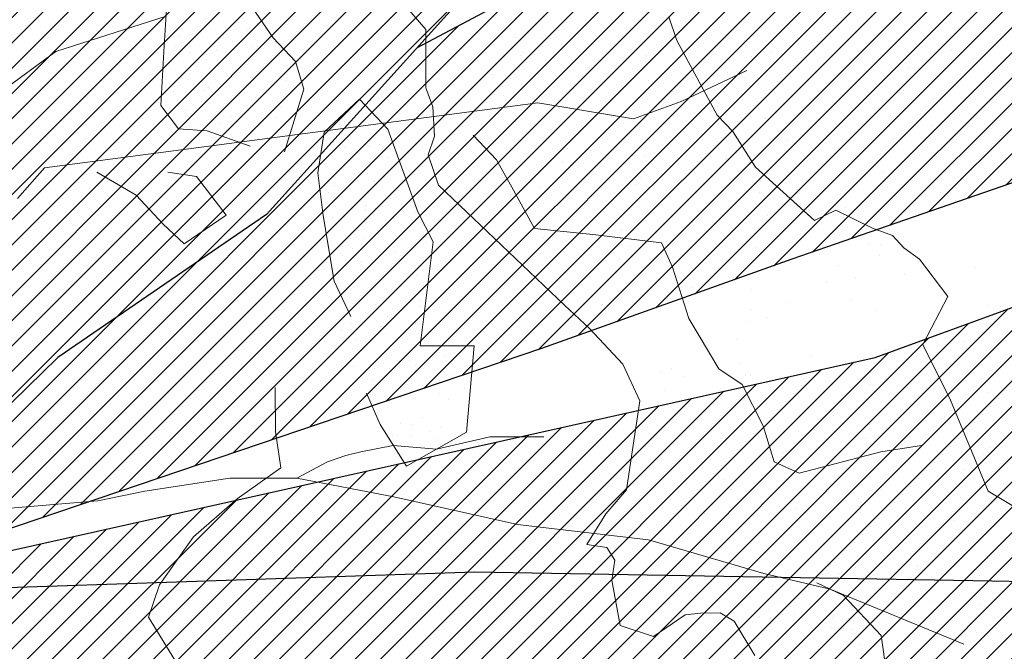
# Model space of a CAD drawing. Units: inches. Extents: x 1986 to 21484, y -1816 to 2016.
# Tile 70 of 85: x 3670.627 to 3679.11, y 1883.347 to 1888.787. Entities that reach past the tile are written whole.
import ezdxf

# ---------------------------------------------------------------- set-up
doc = ezdxf.new("R2010")
doc.units = ezdxf.units.IN
doc.layers.add('L-PLNT', color=84, linetype='Continuous', lineweight=13)
doc.layers.add('vfolhas', color=114, linetype='Continuous', lineweight=5)
doc.layers.add('vfolha2', color=110, linetype='Continuous')
doc.layers.add('vfolhas2', color=102, linetype='Continuous')
pattern_1 = [(45, (-2446.5133113, 50.986076), (-0.004419417382, 0.004419417382), [])]

# ---------------------------------------------------------------- blocks, each defined once
blk = doc.blocks.new('arbusto_PB_verde_grande')
at = {"layer": 'vfolha2'}
h = blk.add_hatch(dxfattribs=at)
h.set_pattern_fill('ANSI31', color=256, scale=0.05, style=0)
h.set_pattern_definition(pattern_1)
h.paths.add_polyline_path([(0.02944, 0.35651), (0.00028, 0.09048), (0.02625, -0.03934), (0.047, 0.06233), (0.06189, 0.09731), (0.09372, 0.26573), (0.09955, 0.43473), (0.08789, 0.61313), (0.0645, 0.72266), (0.04988, 0.6851), (0.0236, 0.51294)])
h.paths.add_polyline_path([(0.30106, 0.43789), (0.14225, 0.24871), (0.26685, 0.30022)])
h.paths.add_polyline_path([(0.37995, 0.22817), (0.23697, 0.15193), (0.18428, 0.09364), (0.11122, 0.04358), (0.02625, -0.03934), (0.28061, 0.04667), (0.36829, 0.07798), (0.46756, 0.11239), (0.61068, 0.19376), (0.71585, 0.27823), (0.55813, 0.25948)])
h.paths.add_polyline_path([(0.56101, -0.29441), (0.72752, -0.32573), (0.59024, -0.2412), (0.42962, -0.15982), (0.02625, -0.03934), (0.14922, -0.14107), (0.18838, -0.16604), (0.41501, -0.24435)])
h.paths.add_polyline_path([(-0.27429, -0.44776), (-0.30352, -0.72628), (-0.23923, -0.64175), (-0.15457, -0.45716), (0.02625, -0.03934), (-0.16328, -0.25376)])
h.paths.add_polyline_path([(-0.51963, -0.24744), (-0.67736, -0.32573), (-0.59558, -0.35072), (-0.40574, -0.32882), (-0.21007, -0.20995), (0.02625, -0.03934), (-0.14874, -0.06595), (-0.31518, -0.09101), (-0.41452, -0.15048)])
h.paths.add_polyline_path([(-0.52546, 0.25007), (-0.70947, 0.24698), (-0.51963, 0.1093), (-0.32979, 0.02167), (-0.07567, -0.0128), (-0.04234, -0.02148), (-0.35024, 0.1312)])
at = {"layer": 'vfolhas'}
h = blk.add_hatch(dxfattribs=at)
h.set_pattern_fill('ANSI31', color=256, scale=0.05, style=0)
h.set_pattern_definition(pattern_1)
h.paths.add_polyline_path([(-0.07279, 0.50669), (-0.18085, 0.65063), (-0.2334, 0.67253), (-0.20712, 0.53176), (-0.10785, 0.25007), (0.02625, -0.03934), (0.00028, 0.09048), (0.00816, 0.16241), (-0.04939, 0.29079)])
h.paths.add_polyline_path([(0.09902, 0.41929), (0.09372, 0.26573), (0.07906, 0.18814), (0.15506, 0.36901), (0.26606, 0.5505), (0.28356, 0.63504), (0.2485, 0.68819), (0.25145, 0.63504), (0.20178, 0.54426)])
h.paths.add_polyline_path([(0.12295, 0.24073), (0.047, 0.06233), (0.02625, -0.03934), (0.11122, 0.04358), (0.18428, 0.09364), (0.27478, 0.19376), (0.3215, 0.25323), (0.44129, 0.38467), (0.47634, 0.57866), (0.41789, 0.45347), (0.28939, 0.30954)])
h.paths.add_polyline_path([(0.58145, -0.03779), (0.70707, 0.01536), (0.78591, 0.04667), (0.74796, 0.06549), (0.62818, 0.08423), (0.52595, 0.09048), (0.39745, 0.04358), (0.02625, -0.03934), (0.25728, -0.03154), (0.43834, -0.0347)])
h.paths.add_polyline_path([(0.52022, -0.03647), (0.43834, -0.0347), (0.25728, -0.03154), (0.02625, -0.03934), (0.17964, -0.08515), (0.53768, -0.13167), (0.69541, -0.15357), (0.78591, -0.07852), (0.70413, -0.10042)])
h.paths.add_polyline_path([(0.27189, -0.21929), (0.14922, -0.14107), (0.02625, -0.03934), (0.15794, -0.31007), (0.29522, -0.42585), (0.41789, -0.49157), (0.56396, -0.56669), (0.5114, -0.48532), (0.39456, -0.34139)])
h.paths.add_polyline_path([(-0.05818, -0.47591), (-0.02312, -0.61984), (0.047, -0.80134), (0.08494, -0.59794), (0.07911, -0.4071), (0.03527, -0.25376), (0.02625, -0.03934), (-0.03773, -0.26001)])
h.paths.add_polyline_path([(-0.24218, 0.14054), (-0.11073, 0.06858), (0.02625, -0.03934), (-0.04235, 0.10871), (-0.21007, 0.23757), (-0.36485, 0.33145), (-0.47874, 0.40341), (-0.54303, 0.46288), (-0.49041, 0.33145), (-0.39408, 0.22192)])
at = {"layer": 'vfolha2'}
for p, q in [((0.23697, 0.15193), (0.37995, 0.22817)), ((0.36829, 0.07798), (0.28061, 0.04667)), ((0.28061, 0.04667), (0.02625, -0.03934))]:
    blk.add_line(p, q, dxfattribs=at)
at = {"layer": 'vfolhas2'}
for p, q in [((0.27478, 0.19376), (0.18428, 0.09364)), ((0.46756, 0.11239), (0.36829, 0.07798)), ((0.18428, 0.09364), (0.11122, 0.04358)), ((0.39745, 0.04358), (0.52595, 0.09048)), ((0.02625, -0.03934), (0.39745, 0.04358)), ((0.11122, 0.04358), (0.02625, -0.03934)), ((0.25728, -0.03154), (0.02625, -0.03934)), ((0.43834, -0.0347), (0.25728, -0.03154)), ((0.58145, -0.03779), (0.43834, -0.0347))]:
    blk.add_line(p, q, dxfattribs=at)
blk = doc.blocks.new('PLANT-SHRUB')
for p, q in [((2157.0668, 1897.0355), (2157.0668, 1897.0355)), ((2157.0784, 1897.0518), (2157.0784, 1897.0518)), ((2157.224, 1897.0515), (2157.739, 1895.9176)), ((2156.8868, 1896.8951), (2156.8868, 1896.8951)), ((2157.4297, 1896.8237), (2157.4297, 1896.8237)), ((2157.6934, 1896.5097), (2157.9487, 1896.8741)), ((2156.5712, 1896.6515), (2156.5712, 1896.6515)), ((2156.6455, 1896.6493), (2156.6455, 1896.6493)), ((2156.7191, 1896.7168), (2156.7191, 1896.7168)), ((2157.159, 1896.6045), (2157.159, 1896.6045)), ((2157.6174, 1896.6382), (2157.6174, 1896.6382)), ((2156.1686, 1896.2344), (2156.0761, 1896.5528)), ((2157.6934, 1896.036), (2157.6934, 1896.5097)), ((2157.875, 1896.4405), (2157.875, 1896.4405)), ((2157.9206, 1896.3661), (2157.9206, 1896.3661)), ((2157.9206, 1896.3661), (2157.9206, 1896.3661)), ((2155.8693, 1895.4412), (2156.1686, 1896.2344)), ((2156.0308, 1896.2768), (2156.0308, 1896.2768)), ((2156.2476, 1896.2848), (2156.2476, 1896.2848)), ((2157.0532, 1896.2817), (2157.0532, 1896.2817)), ((2157.8469, 1896.2986), (2157.8469, 1896.2986)), ((2157.8469, 1896.2986), (2157.8469, 1896.2986)), ((2157.8874, 1896.246), (2157.8874, 1896.246)), ((2157.9914, 1896.2323), (2157.9914, 1896.2323)), ((2158.0927, 1896.2986), (2158.0927, 1896.2986)), ((2158.1327, 1896.2428), (2158.1327, 1896.2428)), ((2158.1327, 1896.2428), (2158.1327, 1896.2428)), ((2158.1327, 1896.2428), (2158.1327, 1896.2428)), ((2156.5523, 1896.218), (2156.5523, 1896.218)), ((2157.7969, 1896.2157), (2157.7969, 1896.2157)), ((2157.7969, 1896.2157), (2157.7969, 1896.2157)), ((2157.9584, 1896.162), (2157.9584, 1896.162)), ((2158.1538, 1896.2109), (2158.1538, 1896.2109)), ((2156.3837, 1896.1106), (2156.3837, 1896.1106)), ((2157.6284, 1896.1083), (2157.6284, 1896.1083)), ((2157.8624, 1896.0555), (2157.8624, 1896.0555)), ((2157.8742, 1896.1083), (2157.8742, 1896.1083)), ((2157.8938, 1896.1163), (2157.8938, 1896.1163)), ((2155.9854, 1895.979), (2155.9854, 1895.979)), ((2157.7846, 1895.7991), (2157.6934, 1896.036)), ((2155.8263, 1895.8987), (2155.8263, 1895.8987)), ((2155.8999, 1895.9662), (2155.8999, 1895.9662)), ((2156.1934, 1895.9516), (2156.1934, 1895.9516)), ((2156.5183, 1895.9088), (2156.5183, 1895.9088)), ((2157.4491, 1895.934), (2157.4491, 1895.934)), ((2157.739, 1895.9176), (2158.063, 1895.429)), ((2158.4945, 1895.9409), (2158.4945, 1895.9409)), ((2158.5295, 1895.5526), (2158.6031, 1895.8917)), ((2156.5461, 1895.8815), (2156.5461, 1895.8815)), ((2157.0612, 1895.8374), (2157.0612, 1895.8374)), ((2157.2692, 1895.81), (2157.2692, 1895.81)), ((2157.5922, 1895.8681), (2157.5922, 1895.8681)), ((2158.1004, 1895.8549), (2158.1004, 1895.8549)), ((2158.1201, 1895.8578), (2158.1201, 1895.8578)), ((2157.5941, 1895.7672), (2157.5941, 1895.7672)), ((2157.9696, 1895.7178), (2157.9696, 1895.7178)), ((2158.2839, 1895.7478), (2158.2839, 1895.7478)), ((2158.3207, 1895.7816), (2158.3207, 1895.7816)), ((2158.137, 1895.6957), (2158.137, 1895.6957)), ((2158.137, 1895.6957), (2158.137, 1895.6957)), ((2158.241, 1895.682), (2158.241, 1895.682)), ((2158.345, 1895.6683), (2158.345, 1895.6683)), ((2158.345, 1895.6683), (2158.345, 1895.6683)), ((2158.345, 1895.6683), (2158.345, 1895.6683)), ((2158.3611, 1895.6729), (2158.3611, 1895.6729)), ((2158.4193, 1895.6605), (2158.4193, 1895.6605)), ((2158.5075, 1895.647), (2158.5075, 1895.647)), ((2155.5916, 1895.606), (2155.5916, 1895.606)), ((2156.32, 1895.5542), (2156.6117, 1895.3538)), ((2156.8362, 1895.6037), (2156.8362, 1895.6037)), ((2157.0277, 1895.5479), (2157.0277, 1895.5479)), ((2157.1014, 1895.6154), (2157.1014, 1895.6154)), ((2158.0809, 1895.6014), (2158.0809, 1895.6014)), ((2158.0809, 1895.6014), (2158.0809, 1895.6014)), ((2158.085, 1895.5656), (2158.085, 1895.5656)), ((2158.3351, 1895.6068), (2158.3351, 1895.6068)), ((2158.5691, 1895.4169), (2158.5295, 1895.5526)), ((2155.4285, 1895.5342), (2155.4285, 1895.5342)), ((2156.0056, 1895.5067), (2156.0056, 1895.5067)), ((2157.028, 1895.5116), (2157.028, 1895.5116)), ((2158.1075, 1895.4727), (2158.1075, 1895.4727)), ((2158.1075, 1895.4727), (2158.1075, 1895.4727)), ((2158.1075, 1895.4727), (2158.1075, 1895.4727)), ((2155.7151, 1894.9276), (2155.8693, 1895.4412)), ((2158.063, 1895.429), (2158.5889, 1894.5368)), ((2158.6936, 1895.3039), (2158.5691, 1895.4169)), ((2156.6117, 1895.3538), (2157.2499, 1895.0076)), ((2158.8011, 1895.2247), (2158.6936, 1895.3039)), ((2155.0808, 1895.2156), (2155.0808, 1895.2156)), ((2156.2295, 1895.2172), (2156.2295, 1895.2172)), ((2157.4741, 1895.2149), (2157.4741, 1895.2149)), ((2158.3029, 1895.2646), (2158.3029, 1895.2646)), ((2158.3029, 1895.2646), (2158.3029, 1895.2646)), ((2158.3485, 1895.2878), (2158.3485, 1895.2878)), ((2159.1292, 1895.1739), (2158.8011, 1895.2247)), ((2155.0071, 1895.1481), (2155.0071, 1895.1481)), ((2155.4414, 1895.1502), (2155.4414, 1895.1502)), ((2156.6299, 1895.1834), (2156.6299, 1895.1834)), ((2158.2292, 1895.1971), (2158.2292, 1895.1971)), ((2158.2292, 1895.1971), (2158.2292, 1895.1971)), ((2158.258, 1895.1601), (2158.258, 1895.1601)), ((2158.3232, 1895.1538), (2158.3232, 1895.1538)), ((2158.475, 1895.1971), (2158.475, 1895.1971)), ((2159.1292, 1895.1739), (2159.1292, 1895.1739)), ((2159.2706, 1894.9082), (2159.1292, 1895.1739)), ((2155.074, 1895.0642), (2155.074, 1895.0642)), ((2156.0609, 1895.1098), (2156.0609, 1895.1098)), ((2156.5209, 1895.1114), (2156.5209, 1895.1114)), ((2157.3056, 1895.1075), (2157.3056, 1895.1075)), ((2157.5671, 1895.098), (2157.5671, 1895.098)), ((2155.6169, 1894.9927), (2155.6169, 1894.9927)), ((2155.8249, 1894.9653), (2155.8249, 1894.9653)), ((2157.2499, 1895.0076), (2157.3411, 1894.7889)), ((2155.2731, 1894.7735), (2155.7151, 1894.9276)), ((2155.7151, 1894.9276), (2155.7151, 1894.9276)), ((2156.1498, 1894.9225), (2156.1498, 1894.9225)), ((2159.0575, 1894.575), (2159.2706, 1894.9082)), ((2156.2086, 1894.7973), (2156.2086, 1894.7973)), ((2156.2822, 1894.8648), (2156.2822, 1894.8648)), ((2156.6927, 1894.8511), (2156.6927, 1894.8511)), ((2156.9007, 1894.8237), (2156.9007, 1894.8237)), ((2157.3411, 1894.7889), (2157.1952, 1894.4974)), ((2157.8314, 1894.8326), (2157.8314, 1894.8326)), ((2154.9343, 1894.75), (2154.9343, 1894.75)), ((2155.232, 1894.373), (2155.2731, 1894.7735)), ((2155.9804, 1894.7366), (2155.9804, 1894.7366)), ((2157.0028, 1894.7415), (2157.0028, 1894.7415)), ((2157.2256, 1894.7809), (2157.2256, 1894.7809)), ((2157.7685, 1894.7094), (2157.7685, 1894.7094)), ((2158.0823, 1894.7026), (2158.0823, 1894.7026)), ((2157.9765, 1894.6821), (2157.9765, 1894.6821)), ((2158.3015, 1894.6393), (2158.3015, 1894.6393)), ((2155.2688, 1894.6051), (2155.2688, 1894.6051)), ((2156.5134, 1894.6029), (2156.5134, 1894.6029)), ((2157.7581, 1894.6006), (2157.7581, 1894.6006)), ((2158.5889, 1894.5368), (2159.3227, 1893.6692)), ((2158.9216, 1894.4663), (2159.0575, 1894.575)), ((2157.1952, 1894.4974), (2157.0858, 1894.1148)), ((2157.41, 1894.4465), (2157.41, 1894.4465)), ((2157.4837, 1894.514), (2157.4837, 1894.514)), ((2158.8944, 1894.3395), (2158.9216, 1894.4663)), ((2154.3938, 1894.3752), (2154.3938, 1894.3752)), ((2155.2628, 1894.2086), (2155.232, 1894.373)), ((2155.4162, 1894.3802), (2155.4162, 1894.3802)), ((2155.8108, 1894.4328), (2155.8108, 1894.4328)), ((2156.4957, 1894.3413), (2156.4957, 1894.3413)), ((2157.5419, 1894.3279), (2157.5419, 1894.3279)), ((2159.0031, 1894.2037), (2158.8944, 1894.3395)), ((2154.6621, 1894.2186), (2154.6621, 1894.2186)), ((2155.2628, 1894.0648), (2155.2628, 1894.2086)), ((2155.9067, 1894.2163), (2155.9067, 1894.2163)), ((2157.1513, 1894.2141), (2157.1513, 1894.2141)), ((2158.7041, 1894.1222), (2159.0031, 1894.2037)), ((2154.1725, 1894.148), (2154.1725, 1894.148)), ((2154.3806, 1894.1207), (2154.3806, 1894.1207)), ((2154.4935, 1894.1112), (2154.4935, 1894.1112)), ((2155.463, 1894.1141), (2155.463, 1894.1141)), ((2155.7382, 1894.109), (2155.7382, 1894.109)), ((2156.9828, 1894.1067), (2156.9828, 1894.1067)), ((2157.0858, 1894.1148), (2157.1405, 1893.878)), ((2158.4322, 1894.0951), (2158.7041, 1894.1222)), ((2154.7055, 1894.0779), (2154.7055, 1894.0779)), ((2155.3451, 1893.9005), (2155.2628, 1894.0648)), ((2155.3894, 1894.0466), (2155.3894, 1894.0466)), ((2157.0122, 1894.082), (2157.0122, 1894.082)), ((2157.8249, 1893.6131), (2158.4322, 1894.0951)), ((2154.9091, 1893.9799), (2154.9091, 1893.9799)), ((2155.2484, 1894.0064), (2155.2484, 1894.0064)), ((2155.4564, 1893.979), (2155.4564, 1893.979)), ((2155.7813, 1893.9362), (2155.7813, 1893.9362)), ((2155.9553, 1893.9665), (2155.9553, 1893.9665)), ((2156.9777, 1893.9714), (2156.9777, 1893.9714)), ((2155.4684, 1893.5718), (2155.3451, 1893.9005)), ((2156.3242, 1893.8648), (2156.3242, 1893.8648)), ((2157.1405, 1893.878), (2157.0311, 1893.386)), ((2158.0571, 1893.9325), (2158.0571, 1893.9325)), ((2156.5322, 1893.8374), (2156.5322, 1893.8374)), ((2156.8571, 1893.7946), (2156.8571, 1893.7946)), ((2154.9916, 1893.6821), (2154.9916, 1893.6821)), ((2156.5908, 1893.6959), (2156.5908, 1893.6959)), ((2156.6645, 1893.7634), (2156.6645, 1893.7634)), ((2157.4, 1893.7231), (2157.4, 1893.7231)), ((2157.608, 1893.6958), (2157.608, 1893.6958)), ((2153.7014, 1893.6066), (2153.7014, 1893.6066)), ((2154.3687, 1893.6052), (2154.3687, 1893.6052)), ((2154.946, 1893.6043), (2154.946, 1893.6043)), ((2155.3911, 1893.6101), (2155.3911, 1893.6101)), ((2156.1906, 1893.6021), (2156.1906, 1893.6021)), ((2157.4353, 1893.5998), (2157.4353, 1893.5998)), ((2157.7148, 1893.2832), (2157.8249, 1893.6131)), ((2157.8249, 1893.6131), (2157.8249, 1893.6131)), ((2157.933, 1893.653), (2157.933, 1893.653)), ((2159.3227, 1893.6692), (2159.9342, 1892.7649)), ((2155.4684, 1893.5718), (2155.4684, 1893.5718)), ((2155.6637, 1893.5102), (2155.4684, 1893.5718)), ((2155.7187, 1892.8278), (2155.6637, 1893.5102)), ((2156.4705, 1893.5712), (2156.4705, 1893.5712)), ((2157.5167, 1893.5578), (2157.5167, 1893.5578)), ((2154.6439, 1893.3635), (2154.6439, 1893.3635)), ((2157.0311, 1893.386), (2156.8305, 1892.967)), ((2154.5702, 1893.296), (2154.5702, 1893.296)), ((2156.193, 1893.3313), (2156.193, 1893.3313)), ((2157.7148, 1893.2832), (2157.7148, 1893.2832)), ((2157.7148, 1892.8616), (2157.7148, 1893.2832)), ((2158.6395, 1893.2743), (2158.9777, 1892.9557)), ((2153.8045, 1893.2487), (2153.8045, 1893.2487)), ((2154.3393, 1893.2178), (2154.3393, 1893.2178)), ((2154.8839, 1893.2098), (2154.8839, 1893.2098)), ((2155.5839, 1893.2155), (2155.5839, 1893.2155)), ((2155.9301, 1893.1964), (2155.9301, 1893.1964)), ((2156.8285, 1893.2133), (2156.8285, 1893.2133)), ((2156.9525, 1893.2013), (2156.9525, 1893.2013)), ((2154.1707, 1893.1104), (2154.1707, 1893.1104)), ((2155.4154, 1893.1082), (2155.4154, 1893.1082)), ((2156.66, 1893.1059), (2156.66, 1893.1059)), ((2155.8453, 1893.0127), (2155.8453, 1893.0127)), ((2154.1724, 1892.9315), (2154.1724, 1892.9315)), ((2155.7717, 1892.9452), (2155.7717, 1892.9452)), ((2156.8305, 1892.967), (2156.7576, 1892.7483)), ((2157.3945, 1892.9806), (2157.3945, 1892.9806)), ((2158.9777, 1892.9557), (2159.3871, 1892.7184)), ((2154.3435, 1892.8351), (2154.3435, 1892.8351)), ((2155.3659, 1892.84), (2155.3659, 1892.84)), ((2157.7331, 1892.5683), (2157.7148, 1892.8616)), ((2155.6536, 1892.4702), (2155.7187, 1892.8278)), ((2156.4454, 1892.8011), (2156.4454, 1892.8011)), ((2156.7576, 1892.7483), (2157.1223, 1892.3111)), ((2157.4915, 1892.7877), (2157.4915, 1892.7877)), ((2158.5418, 1892.2911), (2159.0987, 1892.788)), ((2159.0987, 1892.788), (2159.6754, 1892.6488)), ((2159.9342, 1892.7649), (2160.4349, 1892.0769)), ((2157.0468, 1892.6619), (2157.0468, 1892.6619)), ((2159.3871, 1892.7184), (2159.6357, 1892.4402)), ((2154.6232, 1892.6035), (2154.6232, 1892.6035)), ((2155.3739, 1892.5807), (2155.3739, 1892.5807)), ((2155.8679, 1892.6013), (2155.8679, 1892.6013)), ((2156.9731, 1892.5944), (2156.9731, 1892.5944)), ((2157.1125, 1892.599), (2157.1125, 1892.599)), ((2159.2337, 1892.601), (2159.2337, 1892.601)), ((2159.3179, 1892.6547), (2159.3179, 1892.6547)), ((2159.6754, 1892.6488), (2159.5959, 1892.2315)), ((2159.6754, 1892.6488), (2159.6754, 1892.6488)), ((2157.8167, 1891.0729), (2157.7331, 1892.5683)), ((2158.8533, 1892.497), (2158.8533, 1892.497)), ((2159.3232, 1892.5664), (2159.3232, 1892.5664)), ((2162.2835, 1892.5519), (2162.1841, 1892.075)), ((2154.8587, 1892.4397), (2154.8587, 1892.4397)), ((2155.6536, 1892.2751), (2155.6536, 1892.4702)), ((2155.9049, 1892.4263), (2155.9049, 1892.4263)), ((2156.9273, 1892.4312), (2156.9273, 1892.4312)), ((2159.0157, 1892.4756), (2159.0157, 1892.4756)), ((2159.2872, 1892.4399), (2159.2872, 1892.4399)), ((2159.3912, 1892.4262), (2159.3912, 1892.4262)), ((2159.4307, 1892.4436), (2159.4307, 1892.4436)), ((2159.4675, 1892.4773), (2159.4675, 1892.4773)), ((2159.6357, 1892.4402), (2159.8763, 1892.2895)), ((2158.8376, 1892.3486), (2158.8376, 1892.3486)), ((2159.0411, 1892.3881), (2159.0411, 1892.3881)), ((2159.4599, 1892.3475), (2159.4599, 1892.3475)), ((2159.5537, 1892.4048), (2159.5537, 1892.4048)), ((2159.5808, 1892.3687), (2159.5808, 1892.3687)), ((2155.0262, 1892.2621), (2155.0262, 1892.2621)), ((2155.4666, 1891.568), (2155.6536, 1892.2751)), ((2157.1223, 1892.3111), (2157.4687, 1891.9102)), ((2158.8799, 1891.9731), (2158.5418, 1892.2911)), ((2159.2318, 1892.2613), (2159.2318, 1892.2613)), ((2159.8763, 1892.2895), (2159.9923, 1892.2219)), ((2154.9525, 1892.1946), (2154.9525, 1892.1946)), ((2155.7995, 1891.9784), (2155.2052, 1892.1705)), ((2155.2611, 1892.2147), (2155.2611, 1892.2147)), ((2156.5058, 1892.2125), (2156.5058, 1892.2125)), ((2156.5753, 1892.2299), (2156.5753, 1892.2299)), ((2157.7504, 1892.2102), (2157.7504, 1892.2102)), ((2158.7875, 1892.188), (2158.7875, 1892.188)), ((2159.1565, 1892.1542), (2159.1565, 1892.1542)), ((2159.3106, 1892.1813), (2159.3106, 1892.1813)), ((2159.5959, 1892.2315), (2159.4964, 1891.9533)), ((2159.9923, 1892.2219), (2160.1469, 1892.1543)), ((2160.1469, 1892.1543), (2160.4349, 1892.0769)), ((2155.0926, 1892.1073), (2155.0926, 1892.1073)), ((2155.3407, 1892.0699), (2155.3407, 1892.0699)), ((2156.3372, 1892.1051), (2156.3372, 1892.1051)), ((2157.5818, 1892.1028), (2157.5818, 1892.1028)), ((2159.0211, 1892.0683), (2159.0211, 1892.0683)), ((2159.0579, 1892.102), (2159.0579, 1892.102)), ((2159.0723, 1892.1006), (2159.0723, 1892.1006)), ((2160.4349, 1892.0769), (2160.8561, 1891.6818)), ((2162.1841, 1892.075), (2161.9255, 1891.9359)), ((2156.4202, 1892.031), (2156.4202, 1892.031)), ((2157.4663, 1892.0176), (2157.4663, 1892.0176)), ((2159.0285, 1892.0031), (2159.0285, 1892.0031)), ((2155.0443, 1891.9637), (2155.0443, 1891.9637)), ((2156.2016, 1891.8037), (2155.7995, 1891.9784)), ((2156.2276, 1891.9113), (2156.2276, 1891.9113)), ((2157.4687, 1891.9102), (2157.3776, 1891.5458)), ((2158.1838, 1891.3968), (2158.8799, 1891.9731)), ((2159.1029, 1891.9467), (2159.1029, 1891.9467)), ((2159.2069, 1891.933), (2159.2069, 1891.933)), ((2159.3694, 1891.9117), (2159.3694, 1891.9117)), ((2160.4737, 1891.916), (2160.2947, 1891.6576)), ((2160.9311, 1891.8564), (2160.4737, 1891.916)), ((2161.9255, 1891.9359), (2161.4283, 1891.8365)), ((2155.5872, 1891.8922), (2155.5872, 1891.8922)), ((2155.7952, 1891.8648), (2155.7952, 1891.8648)), ((2156.1202, 1891.822), (2156.1202, 1891.822)), ((2156.1539, 1891.8438), (2156.1539, 1891.8438)), ((2158.8222, 1891.886), (2158.8222, 1891.886)), ((2159.2985, 1891.8471), (2159.2985, 1891.8471)), ((2161.4283, 1891.8365), (2160.9311, 1891.8564)), ((2156.7085, 1891.14), (2156.2016, 1891.8037)), ((2156.663, 1891.7506), (2156.663, 1891.7506)), ((2158.7749, 1891.8029), (2158.7749, 1891.8029)), ((2159.298, 1891.7963), (2159.298, 1891.7963)), ((2155.8797, 1891.6562), (2155.8797, 1891.6562)), ((2156.8711, 1891.7232), (2156.8711, 1891.7232)), ((2156.9021, 1891.6611), (2156.9021, 1891.6611)), ((2157.196, 1891.6804), (2157.196, 1891.6804)), ((2158.6115, 1891.6929), (2158.6115, 1891.6929)), ((2158.6484, 1891.7267), (2158.6484, 1891.7267)), ((2158.9952, 1891.6538), (2158.9952, 1891.6538)), ((2159.4229, 1891.7106), (2159.4229, 1891.7106)), ((2160.2947, 1891.6576), (2160.0361, 1891.3794)), ((2160.8561, 1891.6818), (2161.4664, 1891.2609)), ((2155.3771, 1891.3729), (2155.4666, 1891.568)), ((2155.5451, 1891.6004), (2155.5451, 1891.6004)), ((2156.7897, 1891.5982), (2156.7897, 1891.5982)), ((2157.4291, 1891.5605), (2157.4291, 1891.5605)), ((2158.5047, 1891.6156), (2158.5047, 1891.6156)), ((2158.9109, 1891.6001), (2158.9109, 1891.6001)), ((2159.0159, 1891.618), (2159.0159, 1891.618)), ((2155.7561, 1891.4793), (2155.7561, 1891.4793)), ((2157.3776, 1891.5458), (2157.3046, 1891.2543)), ((2157.3554, 1891.493), (2157.3554, 1891.493)), ((2158.3808, 1891.5244), (2158.3808, 1891.5244)), ((2158.4126, 1891.5107), (2158.4126, 1891.5107)), ((2158.4848, 1891.5107), (2158.4848, 1891.5107)), ((2158.6472, 1891.4893), (2158.6472, 1891.4893)), ((2159.2123, 1891.5176), (2159.2123, 1891.5176)), ((2159.2491, 1891.5513), (2159.2491, 1891.5513)), ((2158.1042, 1891.1186), (2158.1838, 1891.3968)), ((2158.7623, 1891.4179), (2158.7623, 1891.4179)), ((2158.9187, 1891.4536), (2158.9187, 1891.4536)), ((2159.0227, 1891.4399), (2159.0227, 1891.4399)), ((2159.1852, 1891.4185), (2159.1852, 1891.4185)), ((2159.2854, 1891.4112), (2159.2854, 1891.4112)), ((2158.2019, 1891.3176), (2158.2019, 1891.3176)), ((2158.2388, 1891.3514), (2158.2388, 1891.3514)), ((2158.5148, 1891.3478), (2158.5148, 1891.3478)), ((2159.0134, 1891.3353), (2159.0134, 1891.3353)), ((2159.1411, 1891.3794), (2159.039, 1891.059)), ((2159.4566, 1891.3828), (2159.4566, 1891.3828)), ((2156.395, 1891.2609), (2156.395, 1891.2609)), ((2157.3046, 1891.2543), (2157.3046, 1890.9628)), ((2158.4921, 1891.2305), (2158.4921, 1891.2305)), ((2159.0033, 1891.233), (2159.0033, 1891.233)), ((2161.4664, 1891.2609), (2161.8188, 1891.0462)), ((2156.183, 1891.2116), (2156.183, 1891.2116)), ((2160.1908, 1888.6391), (2156.7085, 1891.14)), ((2158.2114, 1891.1546), (2158.2114, 1891.1546)), ((2158.8027, 1891.1422), (2158.8027, 1891.1422)), ((2158.8338, 1891.1534), (2158.8338, 1891.1534)), ((2158.8395, 1891.176), (2158.8395, 1891.176)), ((2156.0144, 1891.1043), (2156.0144, 1891.1043)), ((2156.9576, 1891.1285), (2156.9576, 1891.1285)), ((2157.2591, 1891.102), (2157.2591, 1891.102)), ((2157.702, 1890.8208), (2157.8167, 1891.0729)), ((2157.8059, 1890.423), (2158.1042, 1891.1186)), ((2158.1272, 1891.1009), (2158.1272, 1891.1009)), ((2158.21, 1891.0523), (2158.21, 1891.0523)), ((2159.039, 1891.059), (2158.7208, 1890.582)), ((2158.7495, 1891.0997), (2158.7495, 1891.0997)), ((2158.1965, 1891.0313), (2158.1965, 1891.0313)), ((2158.3005, 1891.0176), (2158.3005, 1891.0176)), ((2158.463, 1890.9962), (2158.463, 1890.9962)), ((2158.7497, 1891.0329), (2158.7497, 1891.0329)), ((2161.8188, 1891.0462), (2163.3587, 1889.8241)), ((2156.877, 1890.8911), (2156.877, 1890.8911)), ((2158.6038, 1890.96), (2158.6038, 1890.96)), ((2158.7344, 1890.9604), (2158.7344, 1890.9604)), ((2158.8385, 1890.9467), (2158.8385, 1890.9467)), ((2156.6099, 1890.8099), (2156.6099, 1890.8099)), ((2157.553, 1890.7406), (2157.702, 1890.8208)), ((2158.3534, 1890.8474), (2158.3534, 1890.8474)), ((2158.4299, 1890.8007), (2158.4299, 1890.8007)), ((2158.4795, 1890.8455), (2158.4795, 1890.8455)), ((2156.2945, 1890.7643), (2156.2945, 1890.7643)), ((2156.5026, 1890.7369), (2156.5026, 1890.7369)), ((2156.5362, 1890.7424), (2156.5362, 1890.7424)), ((2157.3924, 1890.5458), (2157.553, 1890.7406)), ((2158.3931, 1890.7669), (2158.3931, 1890.7669)), ((2156.8275, 1890.6941), (2156.8275, 1890.6941)), ((2158.0501, 1890.6541), (2158.0501, 1890.6541)), ((2158.1974, 1890.6673), (2158.1974, 1890.6673)), ((2158.6724, 1890.653), (2158.6724, 1890.653)), ((2158.7371, 1890.6478), (2158.7371, 1890.6478)), ((2156.4669, 1890.5974), (2156.4669, 1890.5974)), ((2157.3236, 1890.3853), (2157.3924, 1890.5458)), ((2157.9658, 1890.6005), (2157.9658, 1890.6005)), ((2158.1942, 1890.5847), (2158.1942, 1890.5847)), ((2158.7208, 1890.582), (2158.502, 1890.2839)), ((2158.5881, 1890.5993), (2158.5881, 1890.5993)), ((2156.3698, 1890.4908), (2156.3698, 1890.4908)), ((2157.9438, 1890.4671), (2157.9438, 1890.4671)), ((2158.0123, 1890.5381), (2158.0123, 1890.5381)), ((2158.1163, 1890.5244), (2158.1163, 1890.5244)), ((2158.2788, 1890.503), (2158.2788, 1890.503)), ((2158.4669, 1890.4604), (2158.4669, 1890.4604)), ((2158.5502, 1890.4673), (2158.5502, 1890.4673)), ((2156.9795, 1890.0186), (2157.3236, 1890.3853)), ((2157.8059, 1890.0653), (2157.8059, 1890.423)), ((2157.9835, 1890.3916), (2157.9835, 1890.3916)), ((2158.0203, 1890.4253), (2158.0203, 1890.4253)), ((2158.192, 1890.347), (2158.192, 1890.347)), ((2158.1848, 1890.2822), (2158.1848, 1890.2822)), ((2158.502, 1890.2839), (2158.2236, 1890.0653)), ((2158.2236, 1890.0653), (2157.8059, 1890.0653)), ((2156.968, 1889.7436), (2156.9795, 1890.0186)), ((2156.9795, 1890.0186), (2156.9795, 1890.0186)), ((2158.0985, 1889.6745), (2158.5877, 1889.9538)), ((2158.5877, 1889.9538), (2158.5877, 1889.9538)), ((2159.2867, 1889.5907), (2159.3286, 1890.0097)), ((2159.3286, 1890.0097), (2159.7619, 1889.9399)), ((2159.7619, 1889.9399), (2159.7759, 1889.6884)), ((2158.7695, 1889.7164), (2158.9512, 1889.3672)), ((2157.9866, 1889.451), (2158.0985, 1889.6745)), ((2158.3496, 1889.6522), (2158.3496, 1889.6522)), ((2158.4418, 1889.6903), (2158.4418, 1889.6903)), ((2159.7759, 1889.6884), (2159.7759, 1889.3532)), ((2158.2653, 1889.5985), (2158.2653, 1889.5985)), ((2159.4404, 1889.3951), (2159.2867, 1889.5907)), ((2157.9866, 1889.1716), (2157.9866, 1889.451)), ((2158.1596, 1889.5121), (2158.1596, 1889.5121)), ((2158.1817, 1889.481), (2158.1817, 1889.481)), ((2158.2857, 1889.4673), (2158.2857, 1889.4673)), ((2158.4482, 1889.4459), (2158.4482, 1889.4459)), ((2158.5765, 1889.4832), (2158.5765, 1889.4832)), ((2158.6994, 1889.4927), (2158.6994, 1889.4927)), ((2158.7196, 1889.4102), (2158.7196, 1889.4102)), ((2158.8236, 1889.3965), (2158.8236, 1889.3965)), ((2158.9512, 1889.3672), (2159.1189, 1889.1856)), ((2158.3658, 1889.2902), (2158.3658, 1889.2902)), ((2158.4026, 1889.3239), (2158.4026, 1889.3239)), ((2158.4292, 1889.3053), (2158.4292, 1889.3053)), ((2158.4916, 1889.3451), (2158.4916, 1889.3451)), ((2158.9404, 1889.3078), (2158.9404, 1889.3078)), ((2159.7759, 1889.3532), (2159.8877, 1888.9761)), ((2159.1189, 1889.1856), (2159.091, 1888.9342)), ((2157.9168, 1888.7107), (2157.9866, 1889.1716)), ((2158.1471, 1889.1271), (2158.1471, 1889.1271)), ((2158.1669, 1889.1079), (2158.1669, 1889.1079)), ((2158.1882, 1889.1518), (2158.1882, 1889.1518)), ((2158.6868, 1889.1076), (2158.6868, 1889.1076)), ((2158.8105, 1889.1507), (2158.8105, 1889.1507)), ((2158.9665, 1889.1148), (2158.9665, 1889.1148)), ((2159.0033, 1889.1485), (2159.0033, 1889.1485)), ((2158.1039, 1889.0981), (2158.1039, 1889.0981)), ((2158.7262, 1889.097), (2158.7262, 1889.097)), ((2157.9974, 1888.9879), (2157.9974, 1888.9879)), ((2158.1015, 1888.9742), (2158.1015, 1888.9742)), ((2158.2639, 1888.9528), (2158.2639, 1888.9528)), ((2159.091, 1888.9342), (2158.7555, 1888.6129)), ((2158.7676, 1888.9325), (2158.7676, 1888.9325)), ((2158.4166, 1888.9203), (2158.4166, 1888.9203)), ((2158.5354, 1888.917), (2158.5354, 1888.917)), ((2158.6394, 1888.9033), (2158.6394, 1888.9033)), ((2158.8018, 1888.882), (2158.8018, 1888.882)), ((2158.9278, 1888.9227), (2158.9278, 1888.9227)), ((2158.3302, 1888.8447), (2158.3302, 1888.8447)), ((2158.5938, 1888.7732), (2158.5938, 1888.7732)), ((2158.9525, 1888.8435), (2158.9525, 1888.8435)), ((2158.5569, 1888.7395), (2158.5569, 1888.7395)), ((2158.6742, 1888.7226), (2158.6742, 1888.7226)), ((2158.7555, 1888.6129), (2158.3082, 1888.1939)), ((2158.5648, 1888.5966), (2158.5648, 1888.5966)), ((2158.6491, 1888.6503), (2158.6491, 1888.6503)), ((2160.5404, 1888.674), (2160.1908, 1888.6391)), ((2159.4328, 1887.9763), (2158.5318, 1888.4034)), ((2159.4328, 1887.9763), (2159.4328, 1887.9763)), ((2160.0096, 1887.9064), (2159.4328, 1887.9763))]:
    blk.add_line(p, q)

msp = doc.modelspace()

# ---------------------------------------------------------------- block references
at = {"layer": 'L-PLNT', "rotation": 223.1883365522388}
msp.add_blockref('PLANT-SHRUB', (3953.27, 4742.9646), dxfattribs=at)
at = {"layer": 'L-PLNT', "xscale": 24.60366729364114, "yscale": 24.60366729364114, "zscale": 24.60366729364114}
msp.add_blockref('arbusto_PB_verde_grande', (3668.2184, 1884.8051), dxfattribs=at)

doc.saveas('drawing.dxf')
